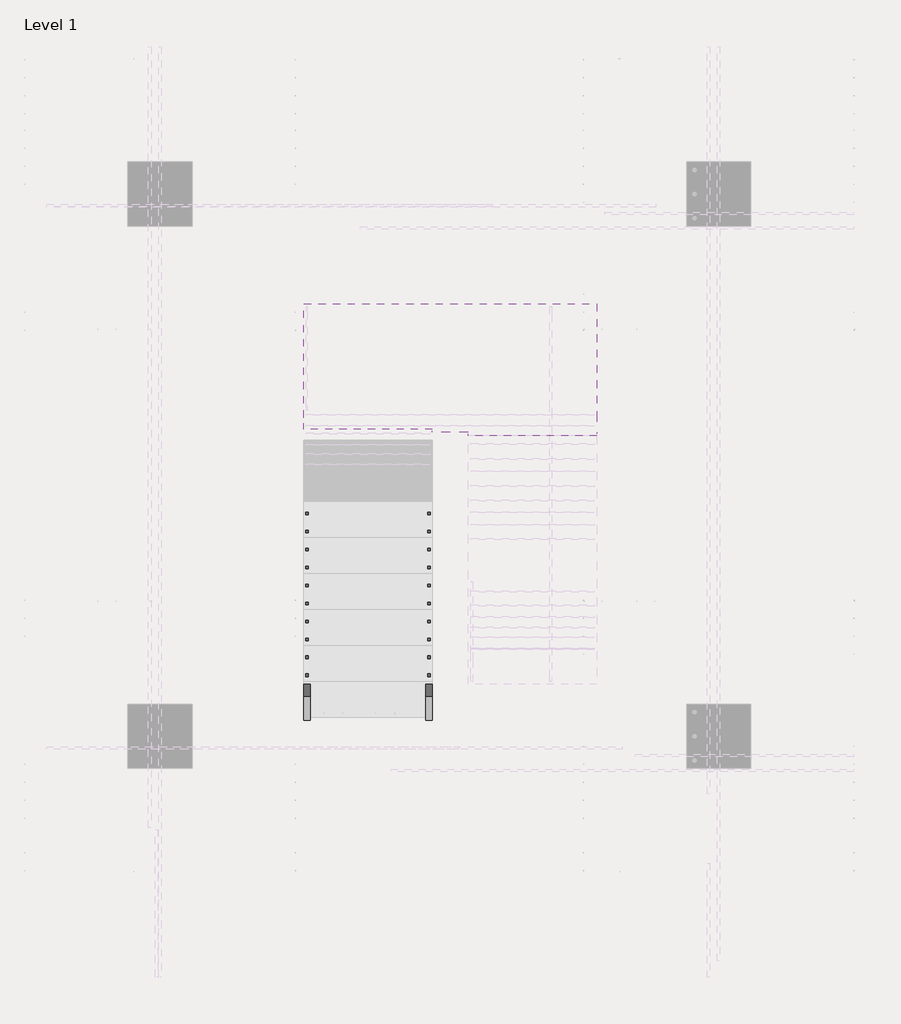
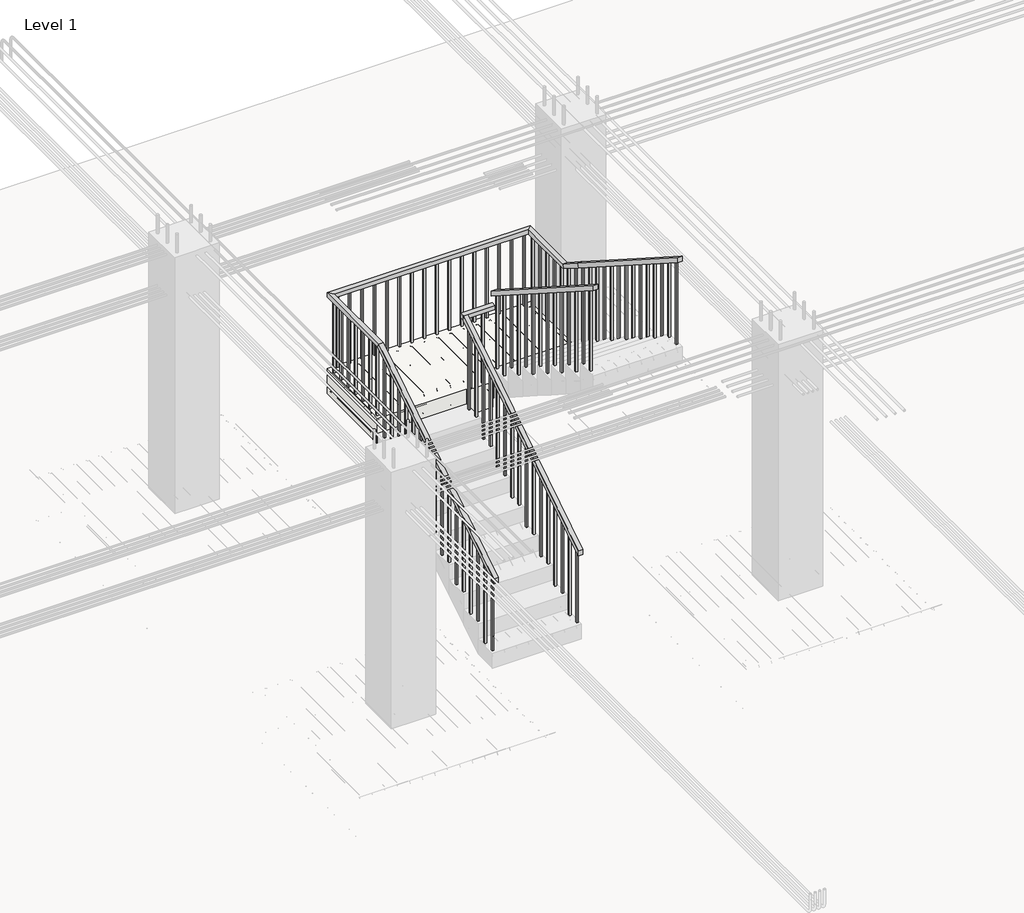
# One storey, part 2 of 17: 2 railings, 1 slab.
"""IFC4 building model written with IfcOpenShell, lengths in millimetres."""

from ifc_helpers import new_model, si_unit, frame, origin, place, context, project, spatial, polyline, outline, extrude, faceted_brep, element, save

model = new_model("IFC4")

# Units and contexts
model_context = context("Model", 3, world=origin())
ifc_project = project(units=[si_unit("LENGTHUNIT", "METRE", prefix="MILLI")], contexts=[model_context])

# Site, building, storey
site = spatial("IfcSite", under=ifc_project)
building = spatial("IfcBuilding", under=site)
storey = spatial("IfcBuildingStorey", under=building, Name="Level 1", Elevation=0.0)

# Railings
placement = place(None, origin())
element("IfcRailing", 1, ObjectType="900mm", at=placement, inside=storey, context=model_context, shape_type="SweptSolid", body=[
    extrude(outline(polyline([(4025.4915698, 1019.9217679), (4025.4915698, 1079.2941176), (6265.8915698, 2513.9031933), (6265.8915698, 2454.5308435), (4025.4915698, 1019.9217679)])), frame((-1977.6746575, 0.0, 0.0), z_axis=(1.0, 0.0, 0.0), x_axis=(0.0, 1.0, 0.0)), (0.0, 0.0, 1.0), 50.0),
    extrude(outline(polyline([(-1977.6746575, 6265.8915698), (-1977.6746575, 6315.8915698), (-1621.8746575, 6315.8915698), (-1621.8746575, 6265.8915698), (-1977.6746575, 6265.8915698)])), frame((0.0, 0.0, 2463.6470588), z_axis=(0.0, 0.0, 1.0), x_axis=(1.0, 0.0, 0.0)), (0.0, 0.0, 1.0), 50.0),
    extrude(outline(polyline([(6290.8915698, 2676.6766387), (6290.8915698, 2617.3042889), (4305.4915698, 3888.6276503), (4305.4915698, 3948.0), (6290.8915698, 2676.6766387)])), frame((-1646.8746575, 0.0, 0.0), z_axis=(1.0, 0.0, 0.0), x_axis=(0.0, 1.0, 0.0)), (0.0, 0.0, 1.0), 50.0),
    extrude(outline(polyline([(4410.8915698, 3821.1362217), (4410.8915698, 2868.7058824), (4390.8915698, 2868.7058824), (4390.8915698, 3833.9429444), (4410.8915698, 3821.1362217)])), frame((-1631.8746575, 0.0, 0.0), z_axis=(1.0, 0.0, 0.0), x_axis=(0.0, 1.0, 0.0)), (0.0, 0.0, 1.0), 20.0),
    extrude(outline(polyline([(4550.8915698, 3731.4891629), (4550.8915698, 2868.7058824), (4530.8915698, 2868.7058824), (4530.8915698, 3744.2958856), (4550.8915698, 3731.4891629)])), frame((-1631.8746575, 0.0, 0.0), z_axis=(1.0, 0.0, 0.0), x_axis=(0.0, 1.0, 0.0)), (0.0, 0.0, 1.0), 20.0),
    extrude(outline(polyline([(4690.8915698, 3641.842104), (4690.8915698, 2689.4117647), (4670.8915698, 2689.4117647), (4670.8915698, 3654.6488267), (4690.8915698, 3641.842104)])), frame((-1631.8746575, 0.0, 0.0), z_axis=(1.0, 0.0, 0.0), x_axis=(0.0, 1.0, 0.0)), (0.0, 0.0, 1.0), 20.0),
    extrude(outline(polyline([(4830.8915698, 3552.1950452), (4830.8915698, 2689.4117647), (4810.8915698, 2689.4117647), (4810.8915698, 3565.0017679), (4830.8915698, 3552.1950452)])), frame((-1631.8746575, 0.0, 0.0), z_axis=(1.0, 0.0, 0.0), x_axis=(0.0, 1.0, 0.0)), (0.0, 0.0, 1.0), 20.0),
    extrude(outline(polyline([(4970.8915698, 3462.5479864), (4970.8915698, 2510.1176471), (4950.8915698, 2510.1176471), (4950.8915698, 3475.3547091), (4970.8915698, 3462.5479864)])), frame((-1631.8746575, 0.0, 0.0), z_axis=(1.0, 0.0, 0.0), x_axis=(0.0, 1.0, 0.0)), (0.0, 0.0, 1.0), 20.0),
    extrude(outline(polyline([(5110.8915698, 3372.9009276), (5110.8915698, 2510.1176471), (5090.8915698, 2510.1176471), (5090.8915698, 3385.7076503), (5110.8915698, 3372.9009276)])), frame((-1631.8746575, 0.0, 0.0), z_axis=(1.0, 0.0, 0.0), x_axis=(0.0, 1.0, 0.0)), (0.0, 0.0, 1.0), 20.0),
    extrude(outline(polyline([(5250.8915698, 3283.2538688), (5250.8915698, 2330.8235294), (5230.8915698, 2330.8235294), (5230.8915698, 3296.0605914), (5250.8915698, 3283.2538688)])), frame((-1631.8746575, 0.0, 0.0), z_axis=(1.0, 0.0, 0.0), x_axis=(0.0, 1.0, 0.0)), (0.0, 0.0, 1.0), 20.0),
    extrude(outline(polyline([(5390.8915698, 3193.6068099), (5390.8915698, 2330.8235294), (5370.8915698, 2330.8235294), (5370.8915698, 3206.4135326), (5390.8915698, 3193.6068099)])), frame((-1631.8746575, 0.0, 0.0), z_axis=(1.0, 0.0, 0.0), x_axis=(0.0, 1.0, 0.0)), (0.0, 0.0, 1.0), 20.0),
    extrude(outline(polyline([(5530.8915698, 3103.9597511), (5530.8915698, 2151.5294118), (5510.8915698, 2151.5294118), (5510.8915698, 3116.7664738), (5530.8915698, 3103.9597511)])), frame((-1631.8746575, 0.0, 0.0), z_axis=(1.0, 0.0, 0.0), x_axis=(0.0, 1.0, 0.0)), (0.0, 0.0, 1.0), 20.0),
    extrude(outline(polyline([(5670.8915698, 3014.3126923), (5670.8915698, 2151.5294118), (5650.8915698, 2151.5294118), (5650.8915698, 3027.119415), (5670.8915698, 3014.3126923)])), frame((-1631.8746575, 0.0, 0.0), z_axis=(1.0, 0.0, 0.0), x_axis=(0.0, 1.0, 0.0)), (0.0, 0.0, 1.0), 20.0),
    extrude(outline(polyline([(5810.8915698, 2924.6656335), (5810.8915698, 1972.2352941), (5790.8915698, 1972.2352941), (5790.8915698, 2937.4723562), (5810.8915698, 2924.6656335)])), frame((-1631.8746575, 0.0, 0.0), z_axis=(1.0, 0.0, 0.0), x_axis=(0.0, 1.0, 0.0)), (0.0, 0.0, 1.0), 20.0),
    extrude(outline(polyline([(5950.8915698, 2835.0185746), (5950.8915698, 1972.2352941), (5930.8915698, 1972.2352941), (5930.8915698, 2847.8252973), (5950.8915698, 2835.0185746)])), frame((-1631.8746575, 0.0, 0.0), z_axis=(1.0, 0.0, 0.0), x_axis=(0.0, 1.0, 0.0)), (0.0, 0.0, 1.0), 20.0),
    extrude(outline(polyline([(6090.8915698, 2745.3715158), (6090.8915698, 1792.9411765), (6070.8915698, 1792.9411765), (6070.8915698, 2758.1782385), (6090.8915698, 2745.3715158)])), frame((-1631.8746575, 0.0, 0.0), z_axis=(1.0, 0.0, 0.0), x_axis=(0.0, 1.0, 0.0)), (0.0, 0.0, 1.0), 20.0),
    extrude(outline(polyline([(6230.8915698, 2655.724457), (6230.8915698, 1792.9411765), (6210.8915698, 1792.9411765), (6210.8915698, 2668.5311797), (6230.8915698, 2655.724457)])), frame((-1631.8746575, 0.0, 0.0), z_axis=(1.0, 0.0, 0.0), x_axis=(0.0, 1.0, 0.0)), (0.0, 0.0, 1.0), 20.0),
    extrude(outline(polyline([(-1752.6746575, 6280.8915698), (-1752.6746575, 6300.8915698), (-1732.6746575, 6300.8915698), (-1732.6746575, 6280.8915698), (-1752.6746575, 6280.8915698)])), frame((0.0, 0.0, 1613.6470588), z_axis=(0.0, 0.0, 1.0), x_axis=(1.0, 0.0, 0.0)), (0.0, 0.0, 1.0), 850.0),
    extrude(outline(polyline([(-1892.6746575, 6280.8915698), (-1892.6746575, 6300.8915698), (-1872.6746575, 6300.8915698), (-1872.6746575, 6280.8915698), (-1892.6746575, 6280.8915698)])), frame((0.0, 0.0, 1613.6470588), z_axis=(0.0, 0.0, 1.0), x_axis=(1.0, 0.0, 0.0)), (0.0, 0.0, 1.0), 850.0),
    extrude(outline(polyline([(6185.4915698, 1434.3529412), (6185.4915698, 2403.0478183), (6205.4915698, 2415.854541), (6205.4915698, 1434.3529412), (6185.4915698, 1434.3529412)])), frame((-1962.6746575, 0.0, 0.0), z_axis=(1.0, 0.0, 0.0), x_axis=(0.0, 1.0, 0.0)), (0.0, 0.0, 1.0), 20.0),
    extrude(outline(polyline([(6045.4915698, 1434.3529412), (6045.4915698, 2313.4007595), (6065.4915698, 2326.2074822), (6065.4915698, 1434.3529412), (6045.4915698, 1434.3529412)])), frame((-1962.6746575, 0.0, 0.0), z_axis=(1.0, 0.0, 0.0), x_axis=(0.0, 1.0, 0.0)), (0.0, 0.0, 1.0), 20.0),
    extrude(outline(polyline([(5905.4915698, 1255.0588235), (5905.4915698, 2223.7537007), (5925.4915698, 2236.5604234), (5925.4915698, 1255.0588235), (5905.4915698, 1255.0588235)])), frame((-1962.6746575, 0.0, 0.0), z_axis=(1.0, 0.0, 0.0), x_axis=(0.0, 1.0, 0.0)), (0.0, 0.0, 1.0), 20.0),
    extrude(outline(polyline([(5765.4915698, 1255.0588235), (5765.4915698, 2134.1066419), (5785.4915698, 2146.9133646), (5785.4915698, 1255.0588235), (5765.4915698, 1255.0588235)])), frame((-1962.6746575, 0.0, 0.0), z_axis=(1.0, 0.0, 0.0), x_axis=(0.0, 1.0, 0.0)), (0.0, 0.0, 1.0), 20.0),
    extrude(outline(polyline([(5625.4915698, 1075.7647059), (5625.4915698, 2044.459583), (5645.4915698, 2057.2663057), (5645.4915698, 1075.7647059), (5625.4915698, 1075.7647059)])), frame((-1962.6746575, 0.0, 0.0), z_axis=(1.0, 0.0, 0.0), x_axis=(0.0, 1.0, 0.0)), (0.0, 0.0, 1.0), 20.0),
    extrude(outline(polyline([(5485.4915698, 1075.7647059), (5485.4915698, 1954.8125242), (5505.4915698, 1967.6192469), (5505.4915698, 1075.7647059), (5485.4915698, 1075.7647059)])), frame((-1962.6746575, 0.0, 0.0), z_axis=(1.0, 0.0, 0.0), x_axis=(0.0, 1.0, 0.0)), (0.0, 0.0, 1.0), 20.0),
    extrude(outline(polyline([(5345.4915698, 896.4705882), (5345.4915698, 1865.1654654), (5365.4915698, 1877.9721881), (5365.4915698, 896.4705882), (5345.4915698, 896.4705882)])), frame((-1962.6746575, 0.0, 0.0), z_axis=(1.0, 0.0, 0.0), x_axis=(0.0, 1.0, 0.0)), (0.0, 0.0, 1.0), 20.0),
    extrude(outline(polyline([(5205.4915698, 896.4705882), (5205.4915698, 1775.5184066), (5225.4915698, 1788.3251293), (5225.4915698, 896.4705882), (5205.4915698, 896.4705882)])), frame((-1962.6746575, 0.0, 0.0), z_axis=(1.0, 0.0, 0.0), x_axis=(0.0, 1.0, 0.0)), (0.0, 0.0, 1.0), 20.0),
    extrude(outline(polyline([(5065.4915698, 717.1764706), (5065.4915698, 1685.8713477), (5085.4915698, 1698.6780704), (5085.4915698, 717.1764706), (5065.4915698, 717.1764706)])), frame((-1962.6746575, 0.0, 0.0), z_axis=(1.0, 0.0, 0.0), x_axis=(0.0, 1.0, 0.0)), (0.0, 0.0, 1.0), 20.0),
    extrude(outline(polyline([(4925.4915698, 717.1764706), (4925.4915698, 1596.2242889), (4945.4915698, 1609.0310116), (4945.4915698, 717.1764706), (4925.4915698, 717.1764706)])), frame((-1962.6746575, 0.0, 0.0), z_axis=(1.0, 0.0, 0.0), x_axis=(0.0, 1.0, 0.0)), (0.0, 0.0, 1.0), 20.0),
    extrude(outline(polyline([(4785.4915698, 537.8823529), (4785.4915698, 1506.5772301), (4805.4915698, 1519.3839528), (4805.4915698, 537.8823529), (4785.4915698, 537.8823529)])), frame((-1962.6746575, 0.0, 0.0), z_axis=(1.0, 0.0, 0.0), x_axis=(0.0, 1.0, 0.0)), (0.0, 0.0, 1.0), 20.0),
    extrude(outline(polyline([(4645.4915698, 537.8823529), (4645.4915698, 1416.9301713), (4665.4915698, 1429.736894), (4665.4915698, 537.8823529), (4645.4915698, 537.8823529)])), frame((-1962.6746575, 0.0, 0.0), z_axis=(1.0, 0.0, 0.0), x_axis=(0.0, 1.0, 0.0)), (0.0, 0.0, 1.0), 20.0),
    extrude(outline(polyline([(4505.4915698, 358.5882353), (4505.4915698, 1327.2831125), (4525.4915698, 1340.0898351), (4525.4915698, 358.5882353), (4505.4915698, 358.5882353)])), frame((-1962.6746575, 0.0, 0.0), z_axis=(1.0, 0.0, 0.0), x_axis=(0.0, 1.0, 0.0)), (0.0, 0.0, 1.0), 20.0),
    extrude(outline(polyline([(4365.4915698, 358.5882353), (4365.4915698, 1237.6360536), (4385.4915698, 1250.4427763), (4385.4915698, 358.5882353), (4365.4915698, 358.5882353)])), frame((-1962.6746575, 0.0, 0.0), z_axis=(1.0, 0.0, 0.0), x_axis=(0.0, 1.0, 0.0)), (0.0, 0.0, 1.0), 20.0),
    extrude(outline(polyline([(4225.4915698, 179.2941176), (4225.4915698, 1147.9889948), (4245.4915698, 1160.7957175), (4245.4915698, 179.2941176), (4225.4915698, 179.2941176)])), frame((-1962.6746575, 0.0, 0.0), z_axis=(1.0, 0.0, 0.0), x_axis=(0.0, 1.0, 0.0)), (0.0, 0.0, 1.0), 20.0),
    extrude(outline(polyline([(4085.4915698, 179.2941176), (4085.4915698, 1058.341936), (4105.4915698, 1071.1486587), (4105.4915698, 179.2941176), (4085.4915698, 179.2941176)])), frame((-1962.6746575, 0.0, 0.0), z_axis=(1.0, 0.0, 0.0), x_axis=(0.0, 1.0, 0.0)), (0.0, 0.0, 1.0), 20.0),
])
element("IfcRailing", 2, ObjectType="900mm", at=placement, inside=storey, context=model_context, shape_type="SolidModel", body=[
    faceted_brep([(-2926.8746575, 4025.4915698, 1079.2941176), (-2926.8746575, 4025.4915698, 1019.9217679), (-2876.8746575, 4025.4915698, 1019.9217679), (-2876.8746575, 4025.4915698, 1079.2941176), (-2926.8746575, 6265.4915698, 2513.6470588), (-2926.8746575, 6280.1281789, 2463.6470588), (-2876.8746575, 6280.1281789, 2463.6470588), (-2876.8746575, 6265.4915698, 2513.6470588), (-2926.8746575, 7265.0915698, 2513.6470588), (-2926.8746575, 7265.0915698, 2463.6470588), (-2876.8746575, 7215.0915698, 2463.6470588), (-2876.8746575, 7215.0915698, 2513.6470588), (-647.6746575, 7265.0915698, 2513.6470588), (-647.6746575, 7265.0915698, 2463.6470588), (-697.6746575, 7215.0915698, 2463.6470588), (-697.6746575, 7215.0915698, 2513.6470588), (-647.6746575, 6545.4915698, 2513.6470588), (-647.6746575, 6530.8549606, 2463.6470588), (-697.6746575, 6530.8549606, 2463.6470588), (-697.6746575, 6545.4915698, 2513.6470588), (-647.6746575, 6265.4915698, 2692.9411765), (-647.6746575, 6238.5288448, 2650.8340338), (-697.6746575, 6238.5288448, 2650.8340338), (-697.6746575, 6265.4915698, 2692.9411765), (-647.6746575, 4305.4915698, 3948.0), (-697.6746575, 4305.4915698, 3948.0), (-697.6746575, 4305.4915698, 3888.6276503), (-647.6746575, 4305.4915698, 3888.6276503)], [[[0, 1, 2, 3]], [[1, 0, 4, 5]], [[2, 1, 5, 6]], [[3, 2, 6, 7]], [[0, 3, 7, 4]], [[5, 4, 8, 9]], [[6, 5, 9, 10]], [[7, 6, 10, 11]], [[4, 7, 11, 8]], [[9, 8, 12, 13]], [[10, 9, 13, 14]], [[11, 10, 14, 15]], [[8, 11, 15, 12]], [[13, 12, 16, 17]], [[14, 13, 17, 18]], [[15, 14, 18, 19]], [[12, 15, 19, 16]], [[17, 16, 20, 21]], [[18, 17, 21, 22]], [[19, 18, 22, 23]], [[16, 19, 23, 20]], [[24, 25, 26, 27]], [[21, 20, 24, 27]], [[22, 21, 27, 26]], [[23, 22, 26, 25]], [[20, 23, 25, 24]]]),
    extrude(outline(polyline([(4385.4915698, 2868.7058824), (4365.4915698, 2868.7058824), (4365.4915698, 3850.2074822), (4385.4915698, 3837.4007595), (4385.4915698, 2868.7058824)])), frame((-682.6746575, 0.0, 0.0), z_axis=(1.0, 0.0, 0.0), x_axis=(0.0, 1.0, 0.0)), (0.0, 0.0, 1.0), 20.0),
    extrude(outline(polyline([(4525.4915698, 2868.7058824), (4505.4915698, 2868.7058824), (4505.4915698, 3760.5604234), (4525.4915698, 3747.7537007), (4525.4915698, 2868.7058824)])), frame((-682.6746575, 0.0, 0.0), z_axis=(1.0, 0.0, 0.0), x_axis=(0.0, 1.0, 0.0)), (0.0, 0.0, 1.0), 20.0),
    extrude(outline(polyline([(4665.4915698, 2689.4117647), (4645.4915698, 2689.4117647), (4645.4915698, 3670.9133646), (4665.4915698, 3658.1066419), (4665.4915698, 2689.4117647)])), frame((-682.6746575, 0.0, 0.0), z_axis=(1.0, 0.0, 0.0), x_axis=(0.0, 1.0, 0.0)), (0.0, 0.0, 1.0), 20.0),
    extrude(outline(polyline([(4805.4915698, 2689.4117647), (4785.4915698, 2689.4117647), (4785.4915698, 3581.2663057), (4805.4915698, 3568.459583), (4805.4915698, 2689.4117647)])), frame((-682.6746575, 0.0, 0.0), z_axis=(1.0, 0.0, 0.0), x_axis=(0.0, 1.0, 0.0)), (0.0, 0.0, 1.0), 20.0),
    extrude(outline(polyline([(4945.4915698, 2510.1176471), (4925.4915698, 2510.1176471), (4925.4915698, 3491.6192469), (4945.4915698, 3478.8125242), (4945.4915698, 2510.1176471)])), frame((-682.6746575, 0.0, 0.0), z_axis=(1.0, 0.0, 0.0), x_axis=(0.0, 1.0, 0.0)), (0.0, 0.0, 1.0), 20.0),
    extrude(outline(polyline([(5085.4915698, 2510.1176471), (5065.4915698, 2510.1176471), (5065.4915698, 3401.9721881), (5085.4915698, 3389.1654654), (5085.4915698, 2510.1176471)])), frame((-682.6746575, 0.0, 0.0), z_axis=(1.0, 0.0, 0.0), x_axis=(0.0, 1.0, 0.0)), (0.0, 0.0, 1.0), 20.0),
    extrude(outline(polyline([(5225.4915698, 2330.8235294), (5205.4915698, 2330.8235294), (5205.4915698, 3312.3251293), (5225.4915698, 3299.5184066), (5225.4915698, 2330.8235294)])), frame((-682.6746575, 0.0, 0.0), z_axis=(1.0, 0.0, 0.0), x_axis=(0.0, 1.0, 0.0)), (0.0, 0.0, 1.0), 20.0),
    extrude(outline(polyline([(5365.4915698, 2330.8235294), (5345.4915698, 2330.8235294), (5345.4915698, 3222.6780704), (5365.4915698, 3209.8713477), (5365.4915698, 2330.8235294)])), frame((-682.6746575, 0.0, 0.0), z_axis=(1.0, 0.0, 0.0), x_axis=(0.0, 1.0, 0.0)), (0.0, 0.0, 1.0), 20.0),
    extrude(outline(polyline([(5505.4915698, 2151.5294118), (5485.4915698, 2151.5294118), (5485.4915698, 3133.0310116), (5505.4915698, 3120.2242889), (5505.4915698, 2151.5294118)])), frame((-682.6746575, 0.0, 0.0), z_axis=(1.0, 0.0, 0.0), x_axis=(0.0, 1.0, 0.0)), (0.0, 0.0, 1.0), 20.0),
    extrude(outline(polyline([(5645.4915698, 2151.5294118), (5625.4915698, 2151.5294118), (5625.4915698, 3043.3839528), (5645.4915698, 3030.5772301), (5645.4915698, 2151.5294118)])), frame((-682.6746575, 0.0, 0.0), z_axis=(1.0, 0.0, 0.0), x_axis=(0.0, 1.0, 0.0)), (0.0, 0.0, 1.0), 20.0),
    extrude(outline(polyline([(5785.4915698, 1972.2352941), (5765.4915698, 1972.2352941), (5765.4915698, 2953.736894), (5785.4915698, 2940.9301713), (5785.4915698, 1972.2352941)])), frame((-682.6746575, 0.0, 0.0), z_axis=(1.0, 0.0, 0.0), x_axis=(0.0, 1.0, 0.0)), (0.0, 0.0, 1.0), 20.0),
    extrude(outline(polyline([(5925.4915698, 1972.2352941), (5905.4915698, 1972.2352941), (5905.4915698, 2864.0898351), (5925.4915698, 2851.2831125), (5925.4915698, 1972.2352941)])), frame((-682.6746575, 0.0, 0.0), z_axis=(1.0, 0.0, 0.0), x_axis=(0.0, 1.0, 0.0)), (0.0, 0.0, 1.0), 20.0),
    extrude(outline(polyline([(6065.4915698, 1792.9411765), (6045.4915698, 1792.9411765), (6045.4915698, 2774.4427763), (6065.4915698, 2761.6360536), (6065.4915698, 1792.9411765)])), frame((-682.6746575, 0.0, 0.0), z_axis=(1.0, 0.0, 0.0), x_axis=(0.0, 1.0, 0.0)), (0.0, 0.0, 1.0), 20.0),
    extrude(outline(polyline([(6205.4915698, 1792.9411765), (6185.4915698, 1792.9411765), (6185.4915698, 2684.7957175), (6205.4915698, 2671.9889948), (6205.4915698, 1792.9411765)])), frame((-682.6746575, 0.0, 0.0), z_axis=(1.0, 0.0, 0.0), x_axis=(0.0, 1.0, 0.0)), (0.0, 0.0, 1.0), 20.0),
    extrude(outline(polyline([(6340.0915698, 1613.6470588), (6320.0915698, 1613.6470588), (6320.0915698, 2598.6064738), (6340.0915698, 2585.7997511), (6340.0915698, 1613.6470588)])), frame((-682.6746575, 0.0, 0.0), z_axis=(1.0, 0.0, 0.0), x_axis=(0.0, 1.0, 0.0)), (0.0, 0.0, 1.0), 20.0),
    extrude(outline(polyline([(6480.0915698, 1613.6470588), (6460.0915698, 1613.6470588), (6460.0915698, 2508.959415), (6480.0915698, 2496.1526923), (6480.0915698, 1613.6470588)])), frame((-682.6746575, 0.0, 0.0), z_axis=(1.0, 0.0, 0.0), x_axis=(0.0, 1.0, 0.0)), (0.0, 0.0, 1.0), 20.0),
    extrude(outline(polyline([(-662.6746575, 6620.0915698), (-662.6746575, 6600.0915698), (-682.6746575, 6600.0915698), (-682.6746575, 6620.0915698), (-662.6746575, 6620.0915698)])), frame((0.0, 0.0, 1613.6470588), z_axis=(0.0, 0.0, 1.0), x_axis=(1.0, 0.0, 0.0)), (0.0, 0.0, 1.0), 850.0),
    extrude(outline(polyline([(-662.6746575, 6760.0915698), (-662.6746575, 6740.0915698), (-682.6746575, 6740.0915698), (-682.6746575, 6760.0915698), (-662.6746575, 6760.0915698)])), frame((0.0, 0.0, 1613.6470588), z_axis=(0.0, 0.0, 1.0), x_axis=(1.0, 0.0, 0.0)), (0.0, 0.0, 1.0), 850.0),
    extrude(outline(polyline([(-662.6746575, 6900.0915698), (-662.6746575, 6880.0915698), (-682.6746575, 6880.0915698), (-682.6746575, 6900.0915698), (-662.6746575, 6900.0915698)])), frame((0.0, 0.0, 1613.6470588), z_axis=(0.0, 0.0, 1.0), x_axis=(1.0, 0.0, 0.0)), (0.0, 0.0, 1.0), 850.0),
    extrude(outline(polyline([(-662.6746575, 7040.0915698), (-662.6746575, 7020.0915698), (-682.6746575, 7020.0915698), (-682.6746575, 7040.0915698), (-662.6746575, 7040.0915698)])), frame((0.0, 0.0, 1613.6470588), z_axis=(0.0, 0.0, 1.0), x_axis=(1.0, 0.0, 0.0)), (0.0, 0.0, 1.0), 850.0),
    extrude(outline(polyline([(-662.6746575, 7180.0915698), (-662.6746575, 7160.0915698), (-682.6746575, 7160.0915698), (-682.6746575, 7180.0915698), (-662.6746575, 7180.0915698)])), frame((0.0, 0.0, 1613.6470588), z_axis=(0.0, 0.0, 1.0), x_axis=(1.0, 0.0, 0.0)), (0.0, 0.0, 1.0), 850.0),
    extrude(outline(polyline([(-741.8746575, 7250.0915698), (-721.8746575, 7250.0915698), (-721.8746575, 7230.0915698), (-741.8746575, 7230.0915698), (-741.8746575, 7250.0915698)])), frame((0.0, 0.0, 1613.6470588), z_axis=(0.0, 0.0, 1.0), x_axis=(1.0, 0.0, 0.0)), (0.0, 0.0, 1.0), 850.0),
    extrude(outline(polyline([(-881.8746575, 7250.0915698), (-861.8746575, 7250.0915698), (-861.8746575, 7230.0915698), (-881.8746575, 7230.0915698), (-881.8746575, 7250.0915698)])), frame((0.0, 0.0, 1613.6470588), z_axis=(0.0, 0.0, 1.0), x_axis=(1.0, 0.0, 0.0)), (0.0, 0.0, 1.0), 850.0),
    extrude(outline(polyline([(-1021.8746575, 7250.0915698), (-1001.8746575, 7250.0915698), (-1001.8746575, 7230.0915698), (-1021.8746575, 7230.0915698), (-1021.8746575, 7250.0915698)])), frame((0.0, 0.0, 1613.6470588), z_axis=(0.0, 0.0, 1.0), x_axis=(1.0, 0.0, 0.0)), (0.0, 0.0, 1.0), 850.0),
    extrude(outline(polyline([(-1161.8746575, 7250.0915698), (-1141.8746575, 7250.0915698), (-1141.8746575, 7230.0915698), (-1161.8746575, 7230.0915698), (-1161.8746575, 7250.0915698)])), frame((0.0, 0.0, 1613.6470588), z_axis=(0.0, 0.0, 1.0), x_axis=(1.0, 0.0, 0.0)), (0.0, 0.0, 1.0), 850.0),
    extrude(outline(polyline([(-1301.8746575, 7250.0915698), (-1281.8746575, 7250.0915698), (-1281.8746575, 7230.0915698), (-1301.8746575, 7230.0915698), (-1301.8746575, 7250.0915698)])), frame((0.0, 0.0, 1613.6470588), z_axis=(0.0, 0.0, 1.0), x_axis=(1.0, 0.0, 0.0)), (0.0, 0.0, 1.0), 850.0),
    extrude(outline(polyline([(-1441.8746575, 7250.0915698), (-1421.8746575, 7250.0915698), (-1421.8746575, 7230.0915698), (-1441.8746575, 7230.0915698), (-1441.8746575, 7250.0915698)])), frame((0.0, 0.0, 1613.6470588), z_axis=(0.0, 0.0, 1.0), x_axis=(1.0, 0.0, 0.0)), (0.0, 0.0, 1.0), 850.0),
    extrude(outline(polyline([(-1581.8746575, 7250.0915698), (-1561.8746575, 7250.0915698), (-1561.8746575, 7230.0915698), (-1581.8746575, 7230.0915698), (-1581.8746575, 7250.0915698)])), frame((0.0, 0.0, 1613.6470588), z_axis=(0.0, 0.0, 1.0), x_axis=(1.0, 0.0, 0.0)), (0.0, 0.0, 1.0), 850.0),
    extrude(outline(polyline([(-1721.8746575, 7250.0915698), (-1701.8746575, 7250.0915698), (-1701.8746575, 7230.0915698), (-1721.8746575, 7230.0915698), (-1721.8746575, 7250.0915698)])), frame((0.0, 0.0, 1613.6470588), z_axis=(0.0, 0.0, 1.0), x_axis=(1.0, 0.0, 0.0)), (0.0, 0.0, 1.0), 850.0),
    extrude(outline(polyline([(-1861.8746575, 7250.0915698), (-1841.8746575, 7250.0915698), (-1841.8746575, 7230.0915698), (-1861.8746575, 7230.0915698), (-1861.8746575, 7250.0915698)])), frame((0.0, 0.0, 1613.6470588), z_axis=(0.0, 0.0, 1.0), x_axis=(1.0, 0.0, 0.0)), (0.0, 0.0, 1.0), 850.0),
    extrude(outline(polyline([(-2001.8746575, 7250.0915698), (-1981.8746575, 7250.0915698), (-1981.8746575, 7230.0915698), (-2001.8746575, 7230.0915698), (-2001.8746575, 7250.0915698)])), frame((0.0, 0.0, 1613.6470588), z_axis=(0.0, 0.0, 1.0), x_axis=(1.0, 0.0, 0.0)), (0.0, 0.0, 1.0), 850.0),
    extrude(outline(polyline([(-2141.8746575, 7250.0915698), (-2121.8746575, 7250.0915698), (-2121.8746575, 7230.0915698), (-2141.8746575, 7230.0915698), (-2141.8746575, 7250.0915698)])), frame((0.0, 0.0, 1613.6470588), z_axis=(0.0, 0.0, 1.0), x_axis=(1.0, 0.0, 0.0)), (0.0, 0.0, 1.0), 850.0),
    extrude(outline(polyline([(-2281.8746575, 7250.0915698), (-2261.8746575, 7250.0915698), (-2261.8746575, 7230.0915698), (-2281.8746575, 7230.0915698), (-2281.8746575, 7250.0915698)])), frame((0.0, 0.0, 1613.6470588), z_axis=(0.0, 0.0, 1.0), x_axis=(1.0, 0.0, 0.0)), (0.0, 0.0, 1.0), 850.0),
    extrude(outline(polyline([(-2421.8746575, 7250.0915698), (-2401.8746575, 7250.0915698), (-2401.8746575, 7230.0915698), (-2421.8746575, 7230.0915698), (-2421.8746575, 7250.0915698)])), frame((0.0, 0.0, 1613.6470588), z_axis=(0.0, 0.0, 1.0), x_axis=(1.0, 0.0, 0.0)), (0.0, 0.0, 1.0), 850.0),
    extrude(outline(polyline([(-2561.8746575, 7250.0915698), (-2541.8746575, 7250.0915698), (-2541.8746575, 7230.0915698), (-2561.8746575, 7230.0915698), (-2561.8746575, 7250.0915698)])), frame((0.0, 0.0, 1613.6470588), z_axis=(0.0, 0.0, 1.0), x_axis=(1.0, 0.0, 0.0)), (0.0, 0.0, 1.0), 850.0),
    extrude(outline(polyline([(-2701.8746575, 7250.0915698), (-2681.8746575, 7250.0915698), (-2681.8746575, 7230.0915698), (-2701.8746575, 7230.0915698), (-2701.8746575, 7250.0915698)])), frame((0.0, 0.0, 1613.6470588), z_axis=(0.0, 0.0, 1.0), x_axis=(1.0, 0.0, 0.0)), (0.0, 0.0, 1.0), 850.0),
    extrude(outline(polyline([(-2841.8746575, 7250.0915698), (-2821.8746575, 7250.0915698), (-2821.8746575, 7230.0915698), (-2841.8746575, 7230.0915698), (-2841.8746575, 7250.0915698)])), frame((0.0, 0.0, 1613.6470588), z_axis=(0.0, 0.0, 1.0), x_axis=(1.0, 0.0, 0.0)), (0.0, 0.0, 1.0), 850.0),
    extrude(outline(polyline([(-2911.8746575, 7165.4915698), (-2911.8746575, 7185.4915698), (-2891.8746575, 7185.4915698), (-2891.8746575, 7165.4915698), (-2911.8746575, 7165.4915698)])), frame((0.0, 0.0, 1613.6470588), z_axis=(0.0, 0.0, 1.0), x_axis=(1.0, 0.0, 0.0)), (0.0, 0.0, 1.0), 850.0),
    extrude(outline(polyline([(-2911.8746575, 7025.4915698), (-2911.8746575, 7045.4915698), (-2891.8746575, 7045.4915698), (-2891.8746575, 7025.4915698), (-2911.8746575, 7025.4915698)])), frame((0.0, 0.0, 1613.6470588), z_axis=(0.0, 0.0, 1.0), x_axis=(1.0, 0.0, 0.0)), (0.0, 0.0, 1.0), 850.0),
    extrude(outline(polyline([(-2911.8746575, 6885.4915698), (-2911.8746575, 6905.4915698), (-2891.8746575, 6905.4915698), (-2891.8746575, 6885.4915698), (-2911.8746575, 6885.4915698)])), frame((0.0, 0.0, 1613.6470588), z_axis=(0.0, 0.0, 1.0), x_axis=(1.0, 0.0, 0.0)), (0.0, 0.0, 1.0), 850.0),
    extrude(outline(polyline([(-2911.8746575, 6745.4915698), (-2911.8746575, 6765.4915698), (-2891.8746575, 6765.4915698), (-2891.8746575, 6745.4915698), (-2911.8746575, 6745.4915698)])), frame((0.0, 0.0, 1613.6470588), z_axis=(0.0, 0.0, 1.0), x_axis=(1.0, 0.0, 0.0)), (0.0, 0.0, 1.0), 850.0),
    extrude(outline(polyline([(-2911.8746575, 6605.4915698), (-2911.8746575, 6625.4915698), (-2891.8746575, 6625.4915698), (-2891.8746575, 6605.4915698), (-2911.8746575, 6605.4915698)])), frame((0.0, 0.0, 1613.6470588), z_axis=(0.0, 0.0, 1.0), x_axis=(1.0, 0.0, 0.0)), (0.0, 0.0, 1.0), 850.0),
    extrude(outline(polyline([(-2911.8746575, 6465.4915698), (-2911.8746575, 6485.4915698), (-2891.8746575, 6485.4915698), (-2891.8746575, 6465.4915698), (-2911.8746575, 6465.4915698)])), frame((0.0, 0.0, 1613.6470588), z_axis=(0.0, 0.0, 1.0), x_axis=(1.0, 0.0, 0.0)), (0.0, 0.0, 1.0), 850.0),
    extrude(outline(polyline([(-2911.8746575, 6325.4915698), (-2911.8746575, 6345.4915698), (-2891.8746575, 6345.4915698), (-2891.8746575, 6325.4915698), (-2911.8746575, 6325.4915698)])), frame((0.0, 0.0, 1613.6470588), z_axis=(0.0, 0.0, 1.0), x_axis=(1.0, 0.0, 0.0)), (0.0, 0.0, 1.0), 850.0),
    extrude(outline(polyline([(6185.4915698, 2403.0478183), (6205.4915698, 2415.854541), (6205.4915698, 1434.3529412), (6185.4915698, 1434.3529412), (6185.4915698, 2403.0478183)])), frame((-2911.8746575, 0.0, 0.0), z_axis=(1.0, 0.0, 0.0), x_axis=(0.0, 1.0, 0.0)), (0.0, 0.0, 1.0), 20.0),
    extrude(outline(polyline([(6045.4915698, 2313.4007595), (6065.4915698, 2326.2074822), (6065.4915698, 1434.3529412), (6045.4915698, 1434.3529412), (6045.4915698, 2313.4007595)])), frame((-2911.8746575, 0.0, 0.0), z_axis=(1.0, 0.0, 0.0), x_axis=(0.0, 1.0, 0.0)), (0.0, 0.0, 1.0), 20.0),
    extrude(outline(polyline([(5905.4915698, 2223.7537007), (5925.4915698, 2236.5604234), (5925.4915698, 1255.0588235), (5905.4915698, 1255.0588235), (5905.4915698, 2223.7537007)])), frame((-2911.8746575, 0.0, 0.0), z_axis=(1.0, 0.0, 0.0), x_axis=(0.0, 1.0, 0.0)), (0.0, 0.0, 1.0), 20.0),
    extrude(outline(polyline([(5765.4915698, 2134.1066419), (5785.4915698, 2146.9133646), (5785.4915698, 1255.0588235), (5765.4915698, 1255.0588235), (5765.4915698, 2134.1066419)])), frame((-2911.8746575, 0.0, 0.0), z_axis=(1.0, 0.0, 0.0), x_axis=(0.0, 1.0, 0.0)), (0.0, 0.0, 1.0), 20.0),
    extrude(outline(polyline([(5625.4915698, 2044.459583), (5645.4915698, 2057.2663057), (5645.4915698, 1075.7647059), (5625.4915698, 1075.7647059), (5625.4915698, 2044.459583)])), frame((-2911.8746575, 0.0, 0.0), z_axis=(1.0, 0.0, 0.0), x_axis=(0.0, 1.0, 0.0)), (0.0, 0.0, 1.0), 20.0),
    extrude(outline(polyline([(5485.4915698, 1954.8125242), (5505.4915698, 1967.6192469), (5505.4915698, 1075.7647059), (5485.4915698, 1075.7647059), (5485.4915698, 1954.8125242)])), frame((-2911.8746575, 0.0, 0.0), z_axis=(1.0, 0.0, 0.0), x_axis=(0.0, 1.0, 0.0)), (0.0, 0.0, 1.0), 20.0),
    extrude(outline(polyline([(5345.4915698, 1865.1654654), (5365.4915698, 1877.9721881), (5365.4915698, 896.4705882), (5345.4915698, 896.4705882), (5345.4915698, 1865.1654654)])), frame((-2911.8746575, 0.0, 0.0), z_axis=(1.0, 0.0, 0.0), x_axis=(0.0, 1.0, 0.0)), (0.0, 0.0, 1.0), 20.0),
    extrude(outline(polyline([(5205.4915698, 1775.5184066), (5225.4915698, 1788.3251293), (5225.4915698, 896.4705882), (5205.4915698, 896.4705882), (5205.4915698, 1775.5184066)])), frame((-2911.8746575, 0.0, 0.0), z_axis=(1.0, 0.0, 0.0), x_axis=(0.0, 1.0, 0.0)), (0.0, 0.0, 1.0), 20.0),
    extrude(outline(polyline([(5065.4915698, 1685.8713477), (5085.4915698, 1698.6780704), (5085.4915698, 717.1764706), (5065.4915698, 717.1764706), (5065.4915698, 1685.8713477)])), frame((-2911.8746575, 0.0, 0.0), z_axis=(1.0, 0.0, 0.0), x_axis=(0.0, 1.0, 0.0)), (0.0, 0.0, 1.0), 20.0),
    extrude(outline(polyline([(4925.4915698, 1596.2242889), (4945.4915698, 1609.0310116), (4945.4915698, 717.1764706), (4925.4915698, 717.1764706), (4925.4915698, 1596.2242889)])), frame((-2911.8746575, 0.0, 0.0), z_axis=(1.0, 0.0, 0.0), x_axis=(0.0, 1.0, 0.0)), (0.0, 0.0, 1.0), 20.0),
    extrude(outline(polyline([(4785.4915698, 1506.5772301), (4805.4915698, 1519.3839528), (4805.4915698, 537.8823529), (4785.4915698, 537.8823529), (4785.4915698, 1506.5772301)])), frame((-2911.8746575, 0.0, 0.0), z_axis=(1.0, 0.0, 0.0), x_axis=(0.0, 1.0, 0.0)), (0.0, 0.0, 1.0), 20.0),
    extrude(outline(polyline([(4645.4915698, 1416.9301713), (4665.4915698, 1429.736894), (4665.4915698, 537.8823529), (4645.4915698, 537.8823529), (4645.4915698, 1416.9301713)])), frame((-2911.8746575, 0.0, 0.0), z_axis=(1.0, 0.0, 0.0), x_axis=(0.0, 1.0, 0.0)), (0.0, 0.0, 1.0), 20.0),
    extrude(outline(polyline([(4505.4915698, 1327.2831125), (4525.4915698, 1340.0898351), (4525.4915698, 358.5882353), (4505.4915698, 358.5882353), (4505.4915698, 1327.2831125)])), frame((-2911.8746575, 0.0, 0.0), z_axis=(1.0, 0.0, 0.0), x_axis=(0.0, 1.0, 0.0)), (0.0, 0.0, 1.0), 20.0),
    extrude(outline(polyline([(4365.4915698, 1237.6360536), (4385.4915698, 1250.4427763), (4385.4915698, 358.5882353), (4365.4915698, 358.5882353), (4365.4915698, 1237.6360536)])), frame((-2911.8746575, 0.0, 0.0), z_axis=(1.0, 0.0, 0.0), x_axis=(0.0, 1.0, 0.0)), (0.0, 0.0, 1.0), 20.0),
    extrude(outline(polyline([(4225.4915698, 1147.9889948), (4245.4915698, 1160.7957175), (4245.4915698, 179.2941176), (4225.4915698, 179.2941176), (4225.4915698, 1147.9889948)])), frame((-2911.8746575, 0.0, 0.0), z_axis=(1.0, 0.0, 0.0), x_axis=(0.0, 1.0, 0.0)), (0.0, 0.0, 1.0), 20.0),
    extrude(outline(polyline([(4085.4915698, 1058.341936), (4105.4915698, 1071.1486587), (4105.4915698, 179.2941176), (4085.4915698, 179.2941176), (4085.4915698, 1058.341936)])), frame((-2911.8746575, 0.0, 0.0), z_axis=(1.0, 0.0, 0.0), x_axis=(0.0, 1.0, 0.0)), (0.0, 0.0, 1.0), 20.0),
])

# Slab
element("IfcSlab", 3, ObjectType="300 mm Thickness", at=placement, inside=storey, context=model_context, shape_type="Brep", body=[
    faceted_brep([(-2927.2746575, 6290.4915698, 1613.6470588), (-1927.2746575, 6290.4915698, 1613.6470588), (-1927.2746575, 6265.4915698, 1613.6470588), (-1647.2746575, 6265.4915698, 1613.6470588), (-1647.2746575, 6240.4915698, 1613.6470588), (-647.2746575, 6240.4915698, 1613.6470588), (-647.2746575, 6265.4915698, 1613.6470588), (-647.2746575, 6430.8337108, 1613.6470588), (-647.2746575, 7265.4915698, 1613.6470588), (-2927.2746575, 7265.4915698, 1613.6470588), (-2927.2746575, 6380.1494288, 1613.6470588), (-2927.2746575, 6290.4915698, 1434.3529412), (-2927.2746575, 6290.4915698, 1256.235892), (-1927.2746575, 6290.4915698, 1256.235892), (-1927.2746575, 6290.4915698, 1313.6470588), (-1927.2746575, 6290.4915698, 1434.3529412), (-1927.2746575, 6265.4915698, 1313.6470588), (-1647.2746575, 6265.4915698, 1313.6470588), (-1647.2746575, 6265.4915698, 1419.5216063), (-1647.2746575, 6240.4915698, 1435.5300096), (-647.2746575, 6240.4915698, 1435.5300096), (-647.2746575, 6265.4915698, 1419.5216063), (-647.2746575, 6430.8337108, 1313.6470588), (-647.2746575, 7265.4915698, 1313.6470588), (-2927.2746575, 7265.4915698, 1313.6470588), (-2927.2746575, 6380.1494288, 1313.6470588), (-1647.2746575, 6430.8337108, 1313.6470588), (-1927.2746575, 6380.1494288, 1313.6470588)], [[[0, 1, 2, 3, 4, 5, 6, 7, 8, 9, 10]], [[1, 0, 11, 12, 13, 14, 15]], [[2, 1, 15, 14, 16]], [[3, 2, 16, 17, 18]], [[4, 3, 18, 19]], [[5, 4, 19, 20]], [[6, 5, 20, 21]], [[6, 21, 22, 23, 8, 7]], [[9, 8, 23, 24]], [[12, 11, 0, 10, 9, 24, 25]], [[26, 17, 16, 14, 27, 25, 24, 23, 22]], [[17, 26, 18]], [[25, 27, 13, 12]], [[27, 14, 13]], [[26, 22, 21, 20, 19, 18]]]),
])

save(model, "model.ifc")

# Revit data of these elements
# Type "900mm"
#   built-in parameter 1008612 = 0.019685 (stored number, unit not read)
#   built-in parameter 1008611 = 0.019685 (stored number, unit not read)
#   built-in parameter 1008609 = 0.902231 (stored number, unit not read)
#   built-in parameter 1008604 = 0.19685 (stored number, unit not read)
#   built-in parameter 1008603 = 0.164042 (stored number, unit not read)
#   Railing Height = 900 mm
#   built-in parameter 1008630 = 2
#   built-in parameter 1008610 = 2
#   built-in parameter 1008608 = 1
#   built-in parameter 1008618 = M_Baluster - Square : 20mm
# Elements 1, 2 (IfcRailing, "900mm")
#   Phase Created = New Construction
# Element 3 (IfcSlab, "300 mm Thickness")
#   Phase Created = New Construction
#   Materials on its faces: "Concrete, Cast In Situ"
# Materials
#   "Concrete, Cast In Situ": class "Concrete", colour RGB 192 192 192, transparency 0, Description = "physical material", Cost = 0
